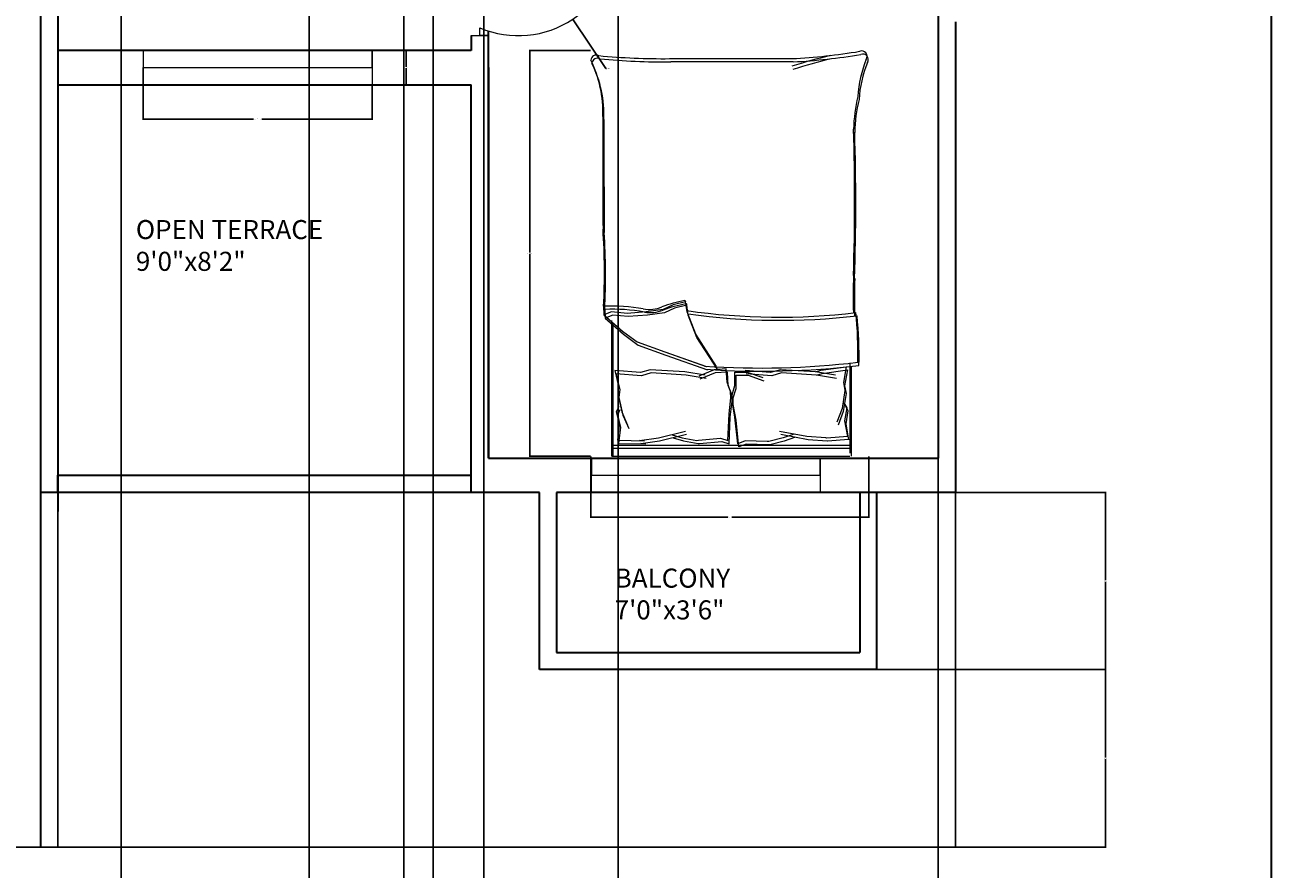
# Model space of a CAD drawing. Units: inches. Extents: x 1734 to 2405, y 1500 to 2491.
# Tile 9 of 14: x 2078 to 2405, y 1700 to 1922. Entities that reach past the tile are written whole.
import ezdxf

# ---------------------------------------------------------------- set-up
doc = ezdxf.new("R2010")
doc.units = ezdxf.units.IN
for name, color, linetype, lineweight in [('A-ANNO-DIMS', 2, 'Continuous', 18), ('A-ANNO-TTLB', 7, 'Continuous', 35), ('A-AREA-IDEN', 7, 'Continuous', 18), ('A-DOOR', 3, 'Continuous', 18), ('A-FURN', 8, 'Continuous', 13), ('A-GLAZ', 4, 'Continuous', 18), ('A-WALL', 7, 'Continuous', 35), ('C-PROP', 7, 'Continuous', 25)]:
    doc.layers.add(name, color=color, linetype=linetype, lineweight=lineweight)
doc.styles.get("Standard").update_dxf_attribs({"font": 'arial.ttf'})
doc.dimstyles.get("Standard").update_dxf_attribs({"dimtxt": 0.18, "dimasz": 0.18, "dimexe": 0.18, "dimexo": 0.0625, "dimgap": 0.09, "dimtad": 0, "dimtih": 1, "dimtoh": 1, "dimdec": 4, "dimzin": 0, "dimdsep": 46, "dimtxsty": 'Standard', "dimcen": 0.09, "dimadec": 0, "dimazin": 0, "dimtfac": 1, "dimtdec": 4, "dimtofl": 0, "dimtmove": 0, "dimatfit": 3, "dimfxl": 1, "dimtolj": 1, "dimtzin": 0, "dimarcsym": 0})

# ---------------------------------------------------------------- blocks, each defined once
blk = doc.blocks.new('BED-DOUBLE')
for p, q in [((81.88, 67.96), (105.53, 67.96)), ((81.88, 67.96), (105.53, 67.96)), ((82.71, 68.26), (106.37, 68.26)), ((82.71, 68.26), (106.37, 68.26)), ((83.83, 60.38), (82.88, 67.03)), ((82.88, 67.03), (87.04, 66.28)), ((83.83, 60.38), (82.88, 67.03)), ((82.88, 67.03), (87.04, 66.28)), ((84.66, 60.68), (83.72, 67.33)), ((83.72, 67.33), (87.87, 66.58)), ((84.66, 60.68), (83.72, 67.33)), ((83.72, 67.33), (87.87, 66.58)), ((87.04, 66.28), (89.12, 66.66)), ((87.04, 66.28), (89.12, 66.66)), ((87.87, 66.58), (89.95, 66.95)), ((87.87, 66.58), (89.95, 66.95)), ((89.12, 66.66), (93.84, 65.9)), ((89.12, 66.66), (93.84, 65.9)), ((89.95, 66.95), (94.67, 66.2)), ((89.95, 66.95), (94.67, 66.2)), ((93.65, 67.22), (92.33, 66.47)), ((93.65, 67.22), (92.33, 66.47)), ((94.48, 67.52), (93.16, 66.77)), ((94.48, 67.52), (93.16, 66.77)), ((97.05, 66.66), (93.65, 67.22)), ((97.05, 66.66), (93.65, 67.22)), ((93.84, 65.9), (97.42, 64.58)), ((93.84, 65.9), (97.42, 64.58)), ((97.88, 66.95), (94.48, 67.52)), ((97.88, 66.95), (94.48, 67.52)), ((94.67, 66.2), (98.26, 64.88)), ((94.67, 66.2), (98.26, 64.88)), ((101.2, 67.41), (97.05, 66.66)), ((101.2, 67.41), (97.05, 66.66)), ((102.04, 67.71), (97.88, 66.95)), ((102.04, 67.71), (97.88, 66.95)), ((101.17, 67.41), (101.6, 61.81)), ((101.17, 67.41), (101.6, 61.82)), ((102.01, 67.7), (102.44, 62.11)), ((102.01, 67.7), (102.44, 62.11)), ((103.53, 67.96), (103.53, 5.54)), ((103.53, 67.96), (103.53, 5.54)), ((104.36, 68.26), (104.36, 5.84)), ((104.36, 68.26), (104.36, 5.84)), ((106.37, 5.54), (106.37, 67.96)), ((85.12, 64.16), (84.25, 58.9)), ((85.12, 64.16), (84.25, 58.9)), ((85.96, 64.46), (85.09, 59.2)), ((85.96, 64.46), (85.09, 59.2)), ((102.44, 62.11), (102.41, 61.98)), ((102.44, 62.11), (102.41, 61.98)), ((84.25, 58.9), (83.69, 49.74)), ((84.25, 58.9), (83.69, 49.74)), ((84.25, 58.9), (83.83, 60.38)), ((84.25, 58.9), (83.83, 60.38)), ((85.09, 59.2), (84.52, 50.04)), ((85.09, 59.2), (84.52, 50.04)), ((85.09, 59.2), (84.66, 60.68)), ((85.09, 59.2), (84.66, 60.68)), ((101.58, 61.68), (101.2, 56.68)), ((101.58, 61.68), (101.2, 56.68)), ((101.6, 61.82), (101.58, 61.68)), ((101.6, 61.81), (101.58, 61.68)), ((102.41, 61.98), (102.04, 56.98)), ((102.41, 61.98), (102.04, 56.98)), ((101.2, 56.68), (99.88, 49.51)), ((101.2, 56.68), (99.88, 49.51)), ((102.04, 56.98), (100.71, 49.81)), ((102.04, 56.98), (100.71, 49.81)), ((2.04, 52.82), (2.04, 20.68)), ((2.04, 52.82), (2.04, 20.68)), ((2.87, 53.12), (2.87, 20.98)), ((2.87, 53.12), (2.87, 20.98)), ((100.64, 53.1), (101.58, 50.45)), ((100.64, 53.1), (101.58, 50.45)), ((101.47, 53.4), (102.41, 50.75)), ((101.47, 53.39), (102.41, 50.75)), ((83.69, 49.74), (84.42, 47.18)), ((83.69, 49.74), (84.42, 47.18)), ((84.52, 50.04), (85.25, 47.48)), ((84.52, 50.04), (85.25, 47.48)), ((101.58, 50.45), (102.52, 46.68)), ((101.58, 50.45), (102.52, 46.68)), ((102.41, 50.75), (103.36, 46.98)), ((102.41, 50.75), (103.36, 46.98)), ((84.42, 47.18), (83.89, 40.48)), ((84.42, 47.18), (83.89, 40.48)), ((85.25, 47.48), (84.72, 40.78)), ((85.25, 47.48), (84.72, 40.78)), ((102.52, 46.26), (102.33, 40.45)), ((102.52, 46.26), (102.33, 40.45)), ((102.52, 46.68), (102.52, 46.26)), ((102.52, 46.68), (102.52, 46.26)), ((103.36, 46.56), (103.17, 40.75)), ((103.36, 46.56), (103.17, 40.75)), ((103.36, 46.98), (103.36, 46.56)), ((103.36, 46.98), (103.36, 46.56)), ((84.29, 41.02), (85.72, 45.13)), ((84.29, 41.02), (85.72, 45.12)), ((85.13, 41.32), (86.55, 45.42)), ((85.13, 41.32), (86.55, 45.42)), ((84.29, 37.81), (84.29, 41.02)), ((84.29, 37.81), (84.29, 41.02)), ((85.13, 38.11), (85.13, 41.32)), ((85.13, 38.11), (85.13, 41.32)), ((102.33, 40.45), (103.09, 38.56)), ((102.33, 40.45), (103.09, 38.56)), ((103.17, 40.75), (103.92, 38.86)), ((103.17, 40.75), (103.92, 38.86)), ((87.79, 37.81), (84.29, 37.81)), ((87.79, 37.81), (84.29, 37.81)), ((87.8, 36.06), (84.3, 35.84)), ((87.8, 36.06), (84.3, 35.84)), ((88.63, 38.11), (85.13, 38.11)), ((88.63, 38.11), (85.13, 38.11)), ((89.37, 36.67), (86.97, 35.76)), ((89.37, 36.67), (86.97, 35.76)), ((90.25, 37.05), (87.79, 37.81)), ((90.25, 37.05), (87.79, 37.81)), ((90.2, 36.96), (87.8, 36.06)), ((90.2, 36.96), (87.8, 36.06)), ((91.08, 37.35), (88.63, 38.11)), ((91.08, 37.35), (88.63, 38.11)), ((91.06, 36.77), (89.37, 36.67)), ((91.06, 36.77), (89.37, 36.67)), ((91.9, 37.07), (90.2, 36.96)), ((91.9, 37.07), (90.2, 36.96)), ((91.95, 37.05), (90.25, 37.05)), ((91.95, 37.05), (90.25, 37.05)), ((95.26, 36.28), (91.06, 36.77)), ((95.26, 36.28), (91.06, 36.77)), ((92.78, 37.35), (91.08, 37.35)), ((92.78, 37.35), (91.08, 37.35)), ((96.09, 36.57), (91.9, 37.07)), ((96.09, 36.58), (91.9, 37.07)), ((96.1, 37.81), (91.95, 37.05)), ((96.1, 37.81), (91.95, 37.05)), ((96.94, 38.11), (92.78, 37.35)), ((96.94, 38.11), (92.78, 37.35)), ((102.28, 35.96), (95.26, 36.28)), ((102.28, 35.96), (95.26, 36.28)), ((103.11, 36.26), (96.09, 36.58)), ((103.11, 36.26), (96.09, 36.57)), ((103.09, 38.56), (96.1, 37.81)), ((103.09, 38.56), (96.1, 37.81)), ((103.92, 38.86), (96.94, 38.11)), ((103.92, 38.86), (96.94, 38.11)), ((102.48, 34.33), (103.11, 36.26)), ((102.48, 34.33), (103.11, 36.26)), ((82.83, 32.98), (74.35, 27.51)), ((82.83, 32.98), (74.35, 27.51)), ((83.66, 33.28), (75.18, 27.8)), ((83.66, 33.28), (75.18, 27.8)), ((86.97, 35.76), (83.47, 35.54)), ((86.97, 35.76), (83.47, 35.54)), ((83.47, 35.54), (83.67, 32.34)), ((83.47, 35.54), (83.67, 32.34)), ((84.3, 35.84), (84.51, 32.63)), ((84.3, 35.84), (84.51, 32.64)), ((101.64, 34.03), (102.28, 35.96)), ((101.64, 34.03), (102.28, 35.96)), ((102.19, 28.24), (101.64, 34.03)), ((102.19, 28.24), (101.64, 34.03)), ((103.03, 28.54), (102.48, 34.33)), ((103.03, 28.54), (102.48, 34.33)), ((79, 19.42), (82.83, 30.31)), ((79, 19.41), (82.83, 30.3)), ((79.83, 19.71), (83.66, 30.6)), ((79.83, 19.71), (83.66, 30.6)), ((83.67, 32.34), (85.35, 28.33)), ((83.67, 32.34), (85.35, 28.33)), ((85.12, 29.97), (84.25, 24.7)), ((85.12, 29.97), (84.25, 24.7)), ((84.51, 32.64), (86.18, 28.63)), ((84.51, 32.63), (86.18, 28.62)), ((85.96, 30.27), (85.09, 25)), ((85.96, 30.27), (85.09, 25)), ((74.35, 27.51), (68.49, 25.28)), ((74.35, 27.51), (68.49, 25.28)), ((75.18, 27.8), (69.32, 25.58)), ((75.18, 27.8), (69.32, 25.58)), ((101.51, 24), (102.22, 27.83)), ((101.51, 24), (102.22, 27.83)), ((102.22, 27.83), (102.19, 28.24)), ((102.22, 27.83), (102.19, 28.24)), ((102.35, 24.3), (103.05, 28.12)), ((102.35, 24.3), (103.05, 28.12)), ((103.05, 28.12), (103.03, 28.54)), ((103.05, 28.12), (103.03, 28.54)), ((68.49, 25.28), (65.86, 24.88)), ((68.49, 25.28), (65.86, 24.88)), ((65.86, 24.88), (66.67, 21.64)), ((65.86, 24.88), (66.67, 21.64)), ((69.32, 25.58), (66.69, 25.17)), ((69.32, 25.58), (66.69, 25.17)), ((66.69, 25.17), (67.5, 21.94)), ((66.69, 25.17), (67.5, 21.94)), ((84.25, 24.7), (83.69, 15.55)), ((84.25, 24.7), (83.69, 15.55)), ((85.09, 25), (84.52, 15.84)), ((85.09, 25), (84.52, 15.85)), ((101.52, 17.76), (99.76, 24.83)), ((101.52, 17.76), (99.76, 24.83)), ((102.36, 18.05), (100.59, 25.13)), ((102.36, 18.05), (100.59, 25.13)), ((100.73, 21.3), (101.51, 24)), ((100.73, 21.3), (101.51, 24)), ((101.57, 21.6), (102.35, 24.3)), ((101.57, 21.6), (102.35, 24.3)), ((66.67, 21.64), (67.88, 19.01)), ((66.67, 21.64), (67.88, 19.01)), ((67.5, 21.94), (68.72, 19.31)), ((67.5, 21.94), (68.72, 19.31)), ((77.21, 12.43), (79.83, 19.71)), ((77.21, 12.43), (79.83, 19.71)), ((67.88, 19.01), (68.49, 14.56)), ((67.88, 19.01), (68.49, 14.56)), ((68.72, 19.31), (69.32, 14.86)), ((68.72, 19.31), (69.32, 14.86)), ((76.37, 12.13), (79, 19.42)), ((76.37, 12.13), (79, 19.41)), ((102.21, 12.8), (101.52, 17.76)), ((102.21, 12.8), (101.52, 17.76)), ((103.05, 13.09), (102.36, 18.05)), ((103.05, 13.09), (102.36, 18.05)), ((68.49, 14.56), (68.89, 9.5)), ((68.49, 14.56), (68.89, 9.5)), ((69.32, 14.86), (69.73, 9.8)), ((69.32, 14.86), (69.73, 9.8)), ((83.69, 15.55), (84.42, 12.99)), ((83.69, 15.55), (84.42, 12.99)), ((84.52, 15.85), (85.25, 13.28)), ((84.52, 15.84), (85.25, 13.28)), ((85.25, 13.28), (84.72, 6.58)), ((85.25, 13.28), (84.72, 6.58)), ((102.19, 7.05), (102.32, 14.11)), ((102.19, 7.05), (102.32, 14.11)), ((102.32, 14.11), (102.21, 12.8)), ((102.32, 14.11), (102.21, 12.8)), ((103.03, 7.35), (103.15, 14.4)), ((103.03, 7.35), (103.15, 14.4)), ((103.15, 14.4), (103.05, 13.09)), ((103.15, 14.4), (103.05, 13.09)), ((73.54, 8.29), (76.37, 12.13)), ((73.54, 8.29), (76.37, 12.13)), ((74.38, 8.59), (77.21, 12.43)), ((74.38, 8.59), (77.21, 12.43)), ((84.42, 12.99), (83.89, 6.28)), ((84.42, 12.99), (83.89, 6.28)), ((95.58, 8.4), (99.08, 9.94)), ((95.58, 8.4), (99.08, 9.94)), ((68.89, 9.5), (68.49, 5.46)), ((68.89, 9.5), (68.49, 5.46)), ((69.3, 3.45), (73.54, 8.29)), ((69.3, 3.45), (73.54, 8.29)), ((69.73, 9.8), (69.32, 5.76)), ((69.73, 9.8), (69.32, 5.76)), ((70.13, 3.75), (74.38, 8.59)), ((70.13, 3.75), (74.38, 8.59)), ((83.89, 6.28), (87.99, 7.3)), ((83.89, 6.28), (87.99, 7.3)), ((84.72, 6.58), (88.82, 7.6)), ((84.72, 6.58), (88.82, 7.59)), ((87.99, 7.3), (90.08, 7.05)), ((87.99, 7.3), (90.08, 7.05)), ((88.82, 7.6), (90.92, 7.35)), ((88.82, 7.59), (90.92, 7.35)), ((90.08, 7.05), (94.75, 8.1)), ((90.08, 7.05), (94.75, 8.1)), ((90.92, 7.35), (95.58, 8.4)), ((90.92, 7.35), (95.58, 8.4)), ((94.64, 6.77), (93.28, 7.44)), ((94.64, 6.77), (93.28, 7.44)), ((95.48, 7.07), (94.11, 7.74)), ((95.48, 7.07), (94.11, 7.74)), ((98, 7.54), (94.64, 6.77)), ((98, 7.54), (94.64, 6.77)), ((94.75, 8.1), (98.25, 9.64)), ((94.75, 8.1), (98.25, 9.64)), ((98.83, 7.84), (95.48, 7.07)), ((98.83, 7.84), (95.48, 7.07)), ((102.19, 7.05), (98, 7.54)), ((102.19, 7.05), (98, 7.54)), ((103.03, 7.35), (98.83, 7.84)), ((103.03, 7.35), (98.83, 7.84)), ((67.02, 3.35), (69.3, 3.45, 5.06)), ((67.02, 3.35), (69.3, 3.45, 5.06)), ((67.85, 3.65), (70.13, 3.75, 5.06)), ((67.85, 3.65), (70.13, 3.75, 5.06)), ((68.49, 5.46), (69.3, 3.45)), ((68.49, 5.46), (69.3, 3.45)), ((69.32, 5.76), (70.13, 3.75)), ((69.32, 5.76), (70.13, 3.75)), ((105.53, 5.54), (70.78, 5.54)), ((105.53, 5.54), (70.78, 5.54)), ((106.37, 5.84), (71.61, 5.84)), ((106.37, 5.84), (71.61, 5.84)), ((106.37, 5.54), (105.53, 5.54))]:
    blk.add_line(p, q)
for centre, radius, start, end in [((1.42, 71.08), 1.42, 56.1736, 203.4781), ((1.42, 71.08), 1.42, 56.1736, 203.4781), ((2.25, 71.38), 1.42, 56.1736, 203.4781), ((2.25, 71.38), 1.42, 56.1736, 203.4781), ((13.75, 100.79), 30.77, 247.9751, 266.652), ((13.75, 100.79), 30.77, 247.9751, 266.652), ((14.58, 101.08), 30.77, 247.9751, 266.652), ((14.58, 101.08), 30.77, 247.9751, 266.652), ((-156.77, 44.51), 159.02, 2.9958, 9.4091), ((-156.77, 44.51), 159.02, 2.9958, 9.4091), ((-155.93, 44.81), 159.02, 2.9958, 9.4091), ((-155.93, 44.81), 159.02, 2.9958, 9.4091), ((21.27, 107.63), 38.7, 256.0648, 268.9113), ((21.27, 107.63), 38.7, 256.0648, 268.9113), ((22.11, 107.93), 38.7, 256.0648, 268.9113), ((22.11, 107.93), 38.7, 256.0648, 268.9113), ((39.43, -560.7), 629.91, 88.22771, 91.71854), ((39.43, -560.7), 629.91, 88.22771, 91.71854), ((40.26, -560.4), 629.91, 88.22771, 91.71854), ((40.26, -560.4), 629.91, 88.22771, 91.71854), ((64.82, 291.01), 222.17, 268.4762, 271.0082), ((64.82, 291.01), 222.17, 268.4762, 271.0082), ((65.65, 291.31), 222.17, 268.4762, 271.0082), ((65.65, 291.31), 222.17, 268.4762, 271.0082), ((-98.62, 49.31), 168.5, 351.7845, 6.9006), ((-98.62, 49.31), 168.5, 351.7845, 6.9006), ((79.29, -38.73), 108.8, 88.7218, 95.604), ((79.29, -38.73), 108.8, 88.7218, 95.604), ((-97.79, 49.61), 168.5, 351.7845, 6.9006), ((-97.79, 49.61), 168.5, 351.7845, 6.9006), ((80.12, -38.43), 108.8, 88.7218, 95.604), ((80.12, -38.43), 108.8, 88.7218, 95.604), ((-132.23, 44.6), 215.46, 356.0865, 6.7821), ((-132.23, 44.6), 215.46, 356.0865, 6.7821), ((-131.4, 44.9), 215.46, 356.0865, 6.7821), ((-131.4, 44.9), 215.46, 356.0865, 6.7821), ((136.5, 94.99), 139.04, 193.3832, 197.7053), ((136.5, 94.99), 139.04, 193.3832, 197.7053), ((137.34, 95.29), 139.04, 193.3832, 197.7053), ((137.34, 95.29), 139.04, 193.3832, 197.7053), ((65.78, 24.65), 0.241, 70.2464, 181.1377), ((65.78, 24.65), 0.241, 70.2464, 181.1377), ((103.6, 31.81), 38.73, 190.6617, 199.8806), ((103.6, 31.81), 38.73, 190.6617, 199.8806), ((66.61, 24.95), 0.241, 70.2464, 181.1377), ((66.61, 24.95), 0.241, 70.2464, 181.1377), ((104.43, 32.11), 38.73, 190.6617, 199.8806), ((104.43, 32.11), 38.73, 190.6617, 199.8806), ((-171.71, 18.75), 173.75, 354.4998, 0.6351), ((-171.71, 18.75), 173.75, 354.4998, 0.6351), ((-170.87, 19.05), 173.75, 354.4998, 0.6351), ((-170.87, 19.05), 173.75, 354.4998, 0.6351), ((59.73, 15.37), 8.13, 348.6608, 23.7384), ((59.73, 15.37), 8.13, 348.6608, 23.7384), ((60.57, 15.67), 8.13, 348.6608, 23.7384), ((60.57, 15.67), 8.13, 348.6608, 23.7384), ((114.23, 5.46), 47.26, 169.8763, 182.5657), ((114.23, 5.46), 47.26, 169.8763, 182.5657), ((115.06, 5.76), 47.26, 169.8763, 182.5657), ((115.06, 5.76), 47.26, 169.8763, 182.5657), ((16.69, -26.67), 30.12, 87.4714, 116.4681), ((16.69, -26.67), 30.12, 87.4714, 116.4681), ((17.79, 5961.38), 5957.95, 270.002168, 270.286887), ((17.79, 5961.38), 5957.95, 270.002168, 270.286887), ((58.1, -165.55), 169.13, 86.9791, 93.8365), ((58.1, -165.55), 169.13, 86.9791, 93.8365), ((58.94, -165.25), 169.13, 86.9791, 93.8365), ((58.94, -165.25), 169.13, 86.9791, 93.8365), ((2.53, 1.44), 1.44, 152.6588, 266.02), ((2.53, 1.44), 1.44, 152.6588, 266.02), ((3.36, 1.73), 1.44, 152.6588, 266.02), ((3.36, 1.74), 1.44, 152.6588, 266.02), ((15.85, -26.97), 30.12, 87.4714, 116.4681), ((15.85, -26.97), 30.12, 87.4714, 116.4681), ((16.96, 5961.08), 5957.95, 270.002168, 270.286887), ((16.96, 5961.08), 5957.95, 270.002168, 270.286887)]:
    blk.add_arc(centre, radius, start, end)
blk = doc.blocks.new('WIN-60-DEEP')
for p, q in [((0, 9), (0, 0)), ((60, 4.5), (60, 9)), ((60, 9), (60, 0)), ((0, 0), (0, 4.5)), ((0, 4.5), (60, 4.5))]:
    blk.add_line(p, q)
blk = doc.blocks.new('*D10')
at = {"layer": 'A-ANNO-DIMS', "color": 0, "lineweight": -2, "transparency": 16777216}
for p, q in [((2226.04, 1914.83), (2209.95, 1914.83)), ((2210.13, 1914.65), (2210.13, 1861.76)), ((2210.13, 1808.5), (2210.13, 1861.4)), ((2226.04, 1808.32), (2209.95, 1808.32))]:
    blk.add_line(p, q, dxfattribs=at)
at = {"layer": 'A-ANNO-DIMS', "color": 0, "transparency": 16777216}
for points in [[(2210.1, 1914.65), (2210.16, 1914.65), (2210.13, 1914.83)], [(2210.1, 1808.5), (2210.16, 1808.5), (2210.13, 1808.32)]]:
    blk.add_solid(points, dxfattribs=at)
at = {"layer": 'Defpoints', "color": 0, "transparency": 16777216}
for p in [(2226.1, 1914.83), (2210.13, 1808.32), (2226.1, 1808.32)]:
    blk.add_point(p, dxfattribs=at)
at = {"layer": 'A-ANNO-DIMS', "color": 0, "transparency": 16777216, "insert": (2210.13, 1861.58), "char_height": 0.18, "attachment_point": 5}
blk.add_mtext('\\A1;BED 107 TYP.', dxfattribs=at)
blk = doc.blocks.new('*D11')
at = {"layer": 'A-ANNO-DIMS', "color": 0, "lineweight": -2, "transparency": 16777216}
for p, q in [((2226.1, 1808.26), (2226.1, 1792.17)), ((2299.01, 1808.26), (2299.01, 1792.17)), ((2226.28, 1792.35), (2262.03, 1792.35)), ((2298.83, 1792.35), (2263.08, 1792.35))]:
    blk.add_line(p, q, dxfattribs=at)
at = {"layer": 'A-ANNO-DIMS', "color": 0, "transparency": 16777216}
for points in [[(2226.28, 1792.38), (2226.28, 1792.32), (2226.1, 1792.35)], [(2298.83, 1792.38), (2298.83, 1792.32), (2299.01, 1792.35)]]:
    blk.add_solid(points, dxfattribs=at)
at = {"layer": 'Defpoints', "color": 0, "transparency": 16777216}
for p in [(2226.1, 1808.32), (2299.01, 1808.32), (2299.01, 1792.35)]:
    blk.add_point(p, dxfattribs=at)
at = {"layer": 'A-ANNO-DIMS', "color": 0, "transparency": 16777216, "insert": (2262.56, 1792.35), "char_height": 0.18, "attachment_point": 5}
blk.add_mtext('\\A1;73 TYP.', dxfattribs=at)
blk = doc.blocks.new('*D18')
at = {"layer": 'A-ANNO-DIMS', "color": 0, "lineweight": -2, "transparency": 16777216}
for p, q in [((2108.7, 1905.76), (2108.7, 1896.64)), ((2168.7, 1905.76), (2168.7, 1896.64)), ((2108.88, 1896.82), (2137.58, 1896.82)), ((2168.52, 1896.82), (2139.82, 1896.82))]:
    blk.add_line(p, q, dxfattribs=at)
at = {"layer": 'A-ANNO-DIMS', "color": 0, "transparency": 16777216}
for points in [[(2108.88, 1896.85), (2108.88, 1896.79), (2108.7, 1896.82)], [(2168.52, 1896.85), (2168.52, 1896.79), (2168.7, 1896.82)]]:
    blk.add_solid(points, dxfattribs=at)
at = {"layer": 'Defpoints', "color": 0, "transparency": 16777216}
for p in [(2108.7, 1905.82), (2168.7, 1905.82), (2168.7, 1896.82)]:
    blk.add_point(p, dxfattribs=at)
at = {"layer": 'A-ANNO-DIMS', "color": 0, "transparency": 16777216, "insert": (2138.7, 1896.82), "char_height": 0.18, "attachment_point": 5}
blk.add_mtext('\\A1;WINDOW 60 TYP.', dxfattribs=at)
blk = doc.blocks.new('*D19')
at = {"layer": 'A-ANNO-DIMS', "color": 0, "lineweight": -2, "transparency": 16777216}
for p, q in [((2168.76, 1914.82), (2177.88, 1914.82)), ((2177.7, 1914.64), (2177.7, 1910.51)), ((2177.7, 1906), (2177.7, 1910.14)), ((2168.76, 1905.82), (2177.88, 1905.82))]:
    blk.add_line(p, q, dxfattribs=at)
at = {"layer": 'A-ANNO-DIMS', "color": 0, "transparency": 16777216}
for points in [[(2177.67, 1914.64), (2177.73, 1914.64), (2177.7, 1914.82)], [(2177.67, 1906), (2177.73, 1906), (2177.7, 1905.82)]]:
    blk.add_solid(points, dxfattribs=at)
at = {"layer": 'Defpoints', "color": 0, "transparency": 16777216}
for p in [(2168.7, 1914.82), (2177.7, 1914.82), (2168.7, 1905.82)]:
    blk.add_point(p, dxfattribs=at)
at = {"layer": 'A-ANNO-DIMS', "color": 0, "transparency": 16777216, "insert": (2177.7, 1910.32), "char_height": 0.18, "attachment_point": 5}
blk.add_mtext('\\A1;9 TYP.', dxfattribs=at)
blk = doc.blocks.new('*D36')
at = {"layer": 'A-ANNO-DIMS', "color": 0, "lineweight": -2, "transparency": 16777216}
for p, q in [((2081.68, 2425.82), (2042.21, 2425.82)), ((2042.39, 2425.64), (2042.39, 2065.96)), ((2042.39, 1705.92), (2042.39, 2065.6)), ((2081.68, 1705.74), (2042.21, 1705.74))]:
    blk.add_line(p, q, dxfattribs=at)
at = {"layer": 'A-ANNO-DIMS', "color": 0, "transparency": 16777216}
for points in [[(2042.36, 2425.64), (2042.42, 2425.64), (2042.39, 2425.82)], [(2042.36, 1705.92), (2042.42, 1705.92), (2042.39, 1705.74)]]:
    blk.add_solid(points, dxfattribs=at)
at = {"layer": 'Defpoints', "color": 0, "transparency": 16777216}
for p in [(2042.39, 2425.82), (2081.74, 2425.82), (2081.74, 1705.74)]:
    blk.add_point(p, dxfattribs=at)
at = {"layer": 'A-ANNO-DIMS', "color": 0, "transparency": 16777216, "insert": (2042.39, 2065.78), "char_height": 0.18, "attachment_point": 5}
blk.add_mtext('\\A1;720.1', dxfattribs=at)
blk = doc.blocks.new('*D37')
at = {"layer": 'A-ANNO-DIMS', "color": 0, "lineweight": -2, "transparency": 16777216}
for p, q in [((2301.2, 1752.32), (2361.27, 1752.32)), ((2361.09, 1752.14), (2361.09, 1729.21)), ((2361.09, 1705.92), (2361.09, 1728.85)), ((2321.81, 1705.74), (2361.27, 1705.74))]:
    blk.add_line(p, q, dxfattribs=at)
at = {"layer": 'A-ANNO-DIMS', "color": 0, "transparency": 16777216}
for points in [[(2361.06, 1752.14), (2361.12, 1752.14), (2361.09, 1752.32)], [(2361.06, 1705.92), (2361.12, 1705.92), (2361.09, 1705.74)]]:
    blk.add_solid(points, dxfattribs=at)
at = {"layer": 'Defpoints', "color": 0, "transparency": 16777216}
for p in [(2301.13, 1752.32), (2361.09, 1752.32), (2321.74, 1705.74)]:
    blk.add_point(p, dxfattribs=at)
at = {"layer": 'A-ANNO-DIMS', "color": 0, "transparency": 16777216, "insert": (2361.09, 1729.03), "char_height": 0.18, "attachment_point": 5}
blk.add_mtext('\\A1;46.58', dxfattribs=at)
blk = doc.blocks.new('*D38')
at = {"layer": 'A-ANNO-DIMS', "color": 0, "lineweight": -2, "transparency": 16777216}
for p, q in [((2321.81, 1798.82), (2361.27, 1798.82)), ((2361.09, 1798.64), (2361.09, 1775.76)), ((2361.09, 1752.5), (2361.09, 1775.39)), ((2301.2, 1752.32), (2361.27, 1752.32))]:
    blk.add_line(p, q, dxfattribs=at)
at = {"layer": 'A-ANNO-DIMS', "color": 0, "transparency": 16777216}
for points in [[(2361.06, 1798.64), (2361.12, 1798.64), (2361.09, 1798.82)], [(2361.06, 1752.5), (2361.12, 1752.5), (2361.09, 1752.32)]]:
    blk.add_solid(points, dxfattribs=at)
at = {"layer": 'Defpoints', "color": 0, "transparency": 16777216}
for p in [(2321.74, 1798.82), (2361.09, 1798.82), (2301.13, 1752.32)]:
    blk.add_point(p, dxfattribs=at)
at = {"layer": 'A-ANNO-DIMS', "color": 0, "transparency": 16777216, "insert": (2361.09, 1775.57), "char_height": 0.18, "attachment_point": 5}
blk.add_mtext('\\A1;46.5', dxfattribs=at)
blk = doc.blocks.new('*D41')
at = {"layer": 'A-ANNO-DIMS', "color": 0, "lineweight": -2, "transparency": 16777216}
for p, q in [((2233.24, 1956.26), (2233.24, 1611.24)), ((2317.24, 1956.26), (2317.24, 1611.24)), ((2233.42, 1611.42), (2275.03, 1611.42)), ((2317.06, 1611.42), (2275.46, 1611.42))]:
    blk.add_line(p, q, dxfattribs=at)
at = {"layer": 'A-ANNO-DIMS', "color": 0, "transparency": 16777216}
for points in [[(2233.42, 1611.45), (2233.42, 1611.39), (2233.24, 1611.42)], [(2317.06, 1611.45), (2317.06, 1611.39), (2317.24, 1611.42)]]:
    blk.add_solid(points, dxfattribs=at)
at = {"layer": 'Defpoints', "color": 0, "transparency": 16777216}
for p in [(2233.24, 1956.32), (2317.24, 1956.32), (2317.24, 1611.42)]:
    blk.add_point(p, dxfattribs=at)
at = {"layer": 'A-ANNO-DIMS', "color": 0, "transparency": 16777216, "insert": (2275.24, 1611.42), "char_height": 0.18, "attachment_point": 5}
blk.add_mtext('\\A1;84', dxfattribs=at)
blk = doc.blocks.new('*D42')
at = {"layer": 'A-ANNO-DIMS', "color": 0, "lineweight": -2, "transparency": 16777216}
for p, q in [((2152.2, 2198.26), (2152.2, 1611.24)), ((2184.72, 2198.26), (2184.72, 1611.24)), ((2152.38, 1611.42), (2168, 1611.42)), ((2184.54, 1611.42), (2168.92, 1611.42))]:
    blk.add_line(p, q, dxfattribs=at)
at = {"layer": 'A-ANNO-DIMS', "color": 0, "transparency": 16777216}
for points in [[(2152.38, 1611.45), (2152.38, 1611.39), (2152.2, 1611.42)], [(2184.54, 1611.45), (2184.54, 1611.39), (2184.72, 1611.42)]]:
    blk.add_solid(points, dxfattribs=at)
at = {"layer": 'Defpoints', "color": 0, "transparency": 16777216}
for p in [(2152.2, 2198.32), (2184.72, 2198.32), (2184.72, 1611.42)]:
    blk.add_point(p, dxfattribs=at)
at = {"layer": 'A-ANNO-DIMS', "color": 0, "transparency": 16777216, "insert": (2168.46, 1611.42), "char_height": 0.18, "attachment_point": 5}
blk.add_mtext('\\A1;32.526', dxfattribs=at)
blk = doc.blocks.new('*D43')
at = {"layer": 'A-ANNO-DIMS', "color": 0, "lineweight": -2, "transparency": 16777216}
for p, q in [((2233.24, 2200.45), (2233.24, 1611.24)), ((2198.08, 2198.26), (2198.08, 1611.24)), ((2198.26, 1611.42), (2215.27, 1611.42)), ((2233.06, 1611.42), (2216.05, 1611.42))]:
    blk.add_line(p, q, dxfattribs=at)
at = {"layer": 'A-ANNO-DIMS', "color": 0, "transparency": 16777216}
for points in [[(2198.26, 1611.45), (2198.26, 1611.39), (2198.08, 1611.42)], [(2233.06, 1611.45), (2233.06, 1611.39), (2233.24, 1611.42)]]:
    blk.add_solid(points, dxfattribs=at)
at = {"layer": 'Defpoints', "color": 0, "transparency": 16777216}
for p in [(2233.24, 2200.51), (2198.08, 2198.32), (2233.24, 1611.42)]:
    blk.add_point(p, dxfattribs=at)
at = {"layer": 'A-ANNO-DIMS', "color": 0, "transparency": 16777216, "insert": (2215.66, 1611.42), "char_height": 0.18, "attachment_point": 5}
blk.add_mtext('\\A1;35.17', dxfattribs=at)
blk = doc.blocks.new('*D44')
at = {"layer": 'A-ANNO-DIMS', "color": 0, "lineweight": -2, "transparency": 16777216}
for p, q in [((2102.87, 2356.76), (2102.87, 1611.24)), ((2177.04, 2356.76), (2177.04, 1611.24)), ((2103.05, 1611.42), (2139.56, 1611.42)), ((2176.86, 1611.42), (2140.35, 1611.42))]:
    blk.add_line(p, q, dxfattribs=at)
at = {"layer": 'A-ANNO-DIMS', "color": 0, "transparency": 16777216}
for points in [[(2103.05, 1611.45), (2103.05, 1611.39), (2102.87, 1611.42)], [(2176.86, 1611.45), (2176.86, 1611.39), (2177.04, 1611.42)]]:
    blk.add_solid(points, dxfattribs=at)
at = {"layer": 'Defpoints', "color": 0, "transparency": 16777216}
for p in [(2102.87, 2356.82), (2177.04, 2356.82), (2177.04, 1611.42)]:
    blk.add_point(p, dxfattribs=at)
at = {"layer": 'A-ANNO-DIMS', "color": 0, "transparency": 16777216, "insert": (2139.96, 1611.42), "char_height": 0.18, "attachment_point": 5}
blk.add_mtext('\\A1;74.17', dxfattribs=at)
blk = doc.blocks.new('*D50')
at = {"layer": 'A-ANNO-DIMS', "color": 0, "lineweight": -2, "transparency": 16777216}
for p, q in [((2206.97, 1944.63), (2207.15, 1944.63)), ((2207.06, 1944.54), (2207.06, 1944.72)), ((2230.01, 1910.06), (2221.5, 1922.88)), ((2230.19, 1910.06), (2230.01, 1910.06))]:
    blk.add_line(p, q, dxfattribs=at)
at = {"layer": 'A-ANNO-DIMS', "color": 0, "transparency": 16777216}
blk.add_solid([(2221.53, 1922.89), (2221.48, 1922.86), (2221.4, 1923.03)], dxfattribs=at)
at = {"layer": 'Defpoints', "color": 0, "transparency": 16777216}
for p in [(2207.06, 1944.63), (2221.4, 1923.03)]:
    blk.add_point(p, dxfattribs=at)
at = {"layer": 'A-ANNO-DIMS', "color": 0, "transparency": 16777216, "insert": (2230.67, 1910.06), "char_height": 0.18, "attachment_point": 5}
blk.add_mtext('\\A1;R25.93', dxfattribs=at)

msp = doc.modelspace()

# ---------------------------------------------------------------- linework, layer by layer
at = {"layer": 'A-ANNO-TTLB'}
msp.add_lwpolyline([(1734.1307, 2491.1293), (2404.5589, 2491.1293), (2404.5589, 1500.293), (1734.1307, 1500.293)], close=True, dxfattribs=at)
at = {"layer": 'A-DOOR'}
for p, q in [((2196.9945, 1918.733), (2196.9945, 1920.733)), ((2194.7445, 1918.733), (2199.2445, 1918.733)), ((2199.2445, 1918.733), (2196.9945, 1918.733))]:
    msp.add_line(p, q, dxfattribs=at)
msp.add_arc((2207.0621, 1944.6313), 25.9324, 247.155856, 0, dxfattribs=at)
at = {"layer": 'A-GLAZ'}
for p, q in [((2226.2942, 1798.8246), (2226.2942, 1807.8246)), ((2226.2942, 1807.8246), (2226.2942, 1803.3246)), ((2286.2942, 1803.3246), (2286.2942, 1807.8246)), ((2286.2942, 1807.8246), (2286.2942, 1798.8246)), ((2226.2942, 1803.3246), (2286.2942, 1803.3246))]:
    msp.add_line(p, q, dxfattribs=at)
at = {"layer": 'A-WALL'}
for p, q in [((2081.7445, 2425.8246), (2081.7445, 1705.7415)), ((2086.2445, 2198.3246), (2086.2445, 1900.8246)), ((2317.2445, 2076.3246), (2317.2445, 1807.8246)), ((2321.7445, 1922.2954), (2321.7445, 1798.8246)), ((2199.2445, 1807.8246), (2199.2445, 1919.9054)), ((2194.7445, 1918.733), (2194.7445, 1914.8246)), ((2194.7445, 1914.8246), (2086.2445, 1914.8246)), ((2199.2445, 1910.3246), (2199.2445, 1807.8246)), ((2086.2445, 1905.8246), (2194.7445, 1905.8246)), ((2086.2445, 1905.8246), (2086.2445, 1793.8246)), ((2194.7445, 1798.8246), (2194.7445, 1905.8246)), ((2317.2445, 1896.3246), (2317.2445, 1807.8246)), ((2199.2445, 1807.8246), (2317.2445, 1807.8246)), ((2086.2445, 1798.8246), (2086.2445, 1803.3246)), ((2086.2445, 1803.3246), (2194.7445, 1803.3246)), ((2194.7445, 1798.8246), (2081.7445, 1798.8246)), ((2212.6326, 1798.8246), (2194.7445, 1798.8246)), ((2212.6326, 1752.3246), (2212.6326, 1798.8246)), ((2321.7445, 1798.8246), (2217.1326, 1798.8246)), ((2217.1326, 1798.8246), (2217.1326, 1756.8246)), ((2301.1326, 1798.8246), (2296.6326, 1798.8246)), ((2296.6326, 1798.8246), (2296.6326, 1756.8246)), ((2301.1326, 1752.3246), (2301.1326, 1798.8246)), ((2217.1326, 1756.8246), (2296.6326, 1756.8246)), ((2217.1326, 1752.3246), (2212.6326, 1752.3246)), ((2301.1326, 1752.3246), (2217.1326, 1752.3246))]:
    msp.add_line(p, q, dxfattribs=at)
at = {"layer": 'C-PROP'}
for p, q in [((2086.2445, 1891.8246), (2086.2445, 1705.7415)), ((2321.7445, 1705.7415), (2321.7445, 1798.8246)), ((2081.7445, 1705.7415), (2321.7445, 1705.7415))]:
    msp.add_line(p, q, dxfattribs=at)

# ---------------------------------------------------------------- block references
at = {"layer": 'A-FURN', "rotation": 270}
msp.add_blockref('BED-DOUBLE', (2226.1022, 1914.6925), dxfattribs=at)
at = {"layer": 'A-GLAZ'}
msp.add_blockref('WIN-60-DEEP', (2108.7017, 1905.825), dxfattribs=at)

# ---------------------------------------------------------------- texts
at = {"layer": 'A-AREA-IDEN', "char_height": 5, "attachment_point": 1}
for s, width, insert in [('OPEN TERRACE\\P9\'0"x8\'2"', 170.000602, (2106.7484, 1870.3044)), ('BALCONY\\P7\'0"x3\'6"', 119.335043, (2232.3611, 1778.8227))]:
    msp.add_mtext_dynamic_manual_height_columns(s, width=width, gutter_width=12.5, heights=[0], dxfattribs=dict(at, insert=insert))

# ---------------------------------------------------------------- dimensions: what is measured, and where the dimension line sits
at = {"layer": 'A-ANNO-DIMS'}
for base, p1, p2, override, picture, middle in [((2042.3945, 2425.8246), (2081.7445, 1705.7415), (2081.7445, 2425.8246), {"dimdec": 1, "dimlfac": 1, "dimrnd": 0, "dimzin": 0, "dimdsep": 46, "dimlunit": 2}, '*D36', (2042.3945, 2065.783)), ((2361.0945, 1798.8246), (2301.1326, 1752.3246), (2321.7445, 1798.8246), {"dimdec": 1, "dimlfac": 1, "dimrnd": 0, "dimzin": 0, "dimdsep": 46, "dimlunit": 2}, '*D38', (2361.0945, 1775.5746)), ((2361.0945, 1752.3246), (2321.7445, 1705.7415), (2301.1326, 1752.3246), {"dimdec": 2, "dimlfac": 1, "dimrnd": 0, "dimzin": 0, "dimdsep": 46, "dimlunit": 2}, '*D37', (2361.0945, 1729.033))]:
    dim = msp.add_linear_dim(base=base, p1=p1, p2=p2, angle=90, dimstyle='Standard', override=override, dxfattribs=at)
    dim.commit()
    dim.dimension.update_dxf_attribs({"geometry": picture, "text_midpoint": middle})
for base, p1, p2, override, picture, middle in [((2177.0411, 1611.4236), (2102.8692, 2356.8246), (2177.0411, 2356.8246), {"dimdec": 2, "dimlfac": 1, "dimrnd": 0, "dimzin": 0, "dimdsep": 46, "dimlunit": 2}, '*D44', (2139.9551, 1611.4236)), ((2233.2445, 1611.4236), (2198.0776, 2198.3246), (2233.2445, 2200.5102), {"dimdec": 2, "dimlfac": 1, "dimrnd": 0, "dimzin": 0, "dimdsep": 46, "dimlunit": 2}, '*D43', (2215.661, 1611.4236)), ((2184.7241, 1611.4236), (2152.1978, 2198.3246), (2184.7241, 2198.3246), {"dimdec": 3, "dimlfac": 1, "dimrnd": 0, "dimzin": 0, "dimdsep": 46, "dimlunit": 2}, '*D42', (2168.461, 1611.4236)), ((2317.2445, 1611.4236), (2233.2445, 1956.3246), (2317.2445, 1956.3246), {"dimdec": 0, "dimlfac": 1, "dimrnd": 0, "dimzin": 0, "dimdsep": 46, "dimlunit": 2}, '*D41', (2275.2445, 1611.4236))]:
    dim = msp.add_linear_dim(base=base, p1=p1, p2=p2, dimstyle='Standard', override=override, dxfattribs=at)
    dim.commit()
    dim.dimension.update_dxf_attribs({"geometry": picture, "text_midpoint": middle})
dim = msp.add_radius_dim(center=(2207.0621, 1944.6313), mpoint=(2221.4048, 1923.0263), dimstyle='Standard', override={"dimdec": 2, "dimlfac": 1, "dimrnd": 0, "dimzin": 0, "dimdsep": 46, "dimlunit": 2}, dxfattribs=at)
dim.commit()
dim.dimension.update_dxf_attribs({"geometry": '*D50', "text_midpoint": (2230.6702, 1910.0633), "dimtype": 164})
for base, p1, p2, angle, text, picture, middle in [((2177.7019, 1914.8246), (2168.7019, 1905.8246), (2168.7019, 1914.8246), 90, '<> TYP.', '*D19', (2177.7019, 1910.3246)), ((2210.1264, 1808.325), (2226.1022, 1914.8304), (2226.1022, 1808.325), 270, 'BED <> TYP.', '*D10', (2210.1264, 1861.5777))]:
    dim = msp.add_linear_dim(base=base, p1=p1, p2=p2, angle=angle, text=text, dimstyle='Standard', override={"dimdec": 0, "dimlfac": 1, "dimrnd": 0, "dimzin": 0, "dimdsep": 46, "dimlunit": 2}, dxfattribs=at)
    dim.commit()
    dim.dimension.update_dxf_attribs({"geometry": picture, "text_midpoint": middle})
for base, p1, p2, text, picture, middle in [((2168.7019, 1896.8246), (2108.7019, 1905.8246), (2168.7019, 1905.8246), 'WINDOW <> TYP.', '*D18', (2138.7019, 1896.8246)), ((2299.0111, 1792.3492), (2226.1022, 1808.325), (2299.0111, 1808.325), '<> TYP.', '*D11', (2262.5567, 1792.3492))]:
    dim = msp.add_linear_dim(base=base, p1=p1, p2=p2, text=text, dimstyle='Standard', override={"dimdec": 0, "dimlfac": 1, "dimrnd": 0, "dimzin": 0, "dimdsep": 46, "dimlunit": 2}, dxfattribs=at)
    dim.commit()
    dim.dimension.update_dxf_attribs({"geometry": picture, "text_midpoint": middle})

doc.saveas('drawing.dxf')
